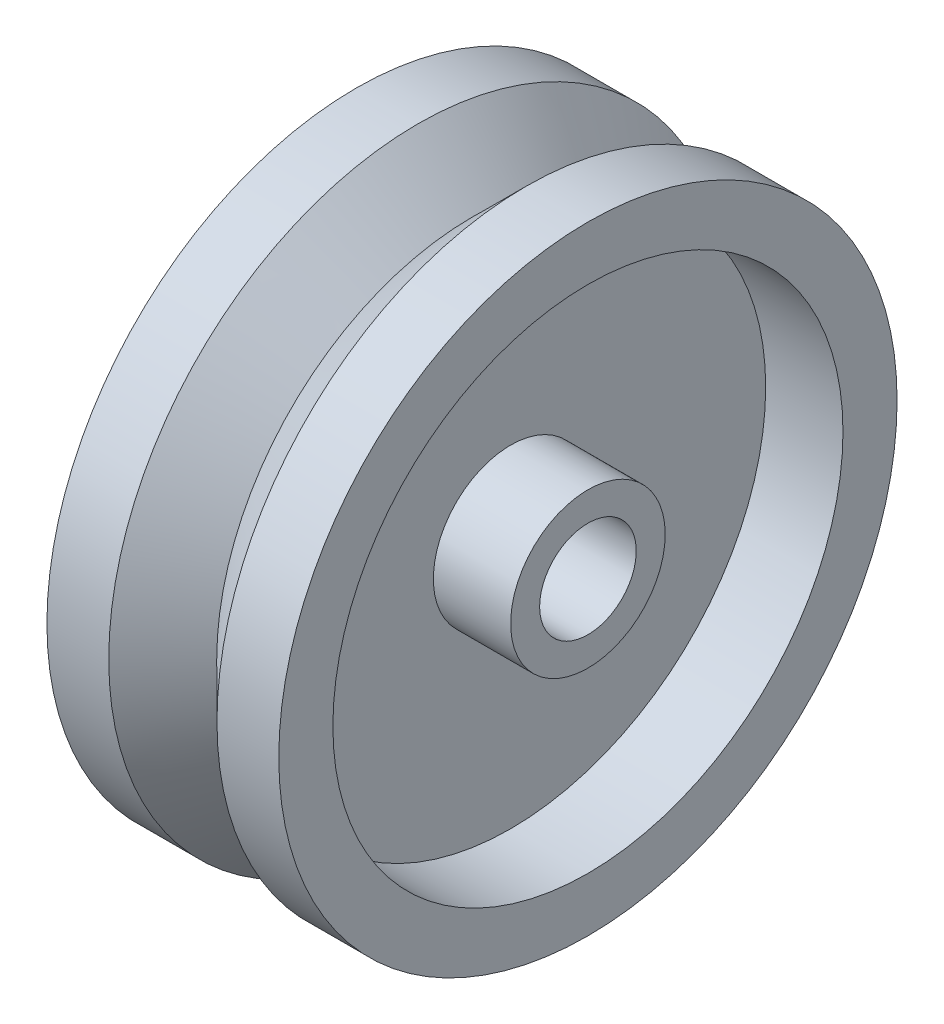
ISO-10303-21;
HEADER;
FILE_DESCRIPTION(('STEP AP214'),'2;1');
FILE_NAME('part.step','',(''),(''),'','','');
FILE_SCHEMA(('AUTOMOTIVE_DESIGN { 1 0 10303 214 1 1 1 1 }'));
ENDSEC;
DATA;
#1=APPLICATION_CONTEXT('core data for automotive mechanical design processes');
#2=APPLICATION_PROTOCOL_DEFINITION('international standard','automotive_design',2000,#1);
#3=PRODUCT_CONTEXT('',#1,'mechanical');
#4=PRODUCT('Part','Part','',(#3));
#5=PRODUCT_RELATED_PRODUCT_CATEGORY('part','',(#4));
#6=PRODUCT_DEFINITION_FORMATION('','',#4);
#7=PRODUCT_DEFINITION_CONTEXT('part definition',#1,'design');
#8=PRODUCT_DEFINITION('design','',#6,#7);
#9=PRODUCT_DEFINITION_SHAPE('','',#8);
#10=(LENGTH_UNIT() NAMED_UNIT(*) SI_UNIT(.MILLI.,.METRE.));
#11=(NAMED_UNIT(*) PLANE_ANGLE_UNIT() SI_UNIT($,.RADIAN.));
#12=(NAMED_UNIT(*) SI_UNIT($,.STERADIAN.) SOLID_ANGLE_UNIT());
#13=UNCERTAINTY_MEASURE_WITH_UNIT(LENGTH_MEASURE(1.E-05),#10,'distance_accuracy_value','');
#14=(GEOMETRIC_REPRESENTATION_CONTEXT(3) GLOBAL_UNCERTAINTY_ASSIGNED_CONTEXT((#13)) GLOBAL_UNIT_ASSIGNED_CONTEXT((#10,
#11,#12)) REPRESENTATION_CONTEXT('',''));
#15=CARTESIAN_POINT('',(0.,0.,0.));
#16=DIRECTION('',(0.,0.,1.));
#17=DIRECTION('',(1.,0.,0.));
#18=AXIS2_PLACEMENT_3D('',#15,#16,#17);
#19=CARTESIAN_POINT('',(-7.5,-3.125,0.));
#20=DIRECTION('',(-1.,0.,0.));
#21=DIRECTION('',(0.,0.,1.));
#22=AXIS2_PLACEMENT_3D('',#19,#20,#21);
#23=PLANE('',#22);
#24=CARTESIAN_POINT('',(-7.5,0.,0.));
#25=DIRECTION('',(-1.,0.,0.));
#26=DIRECTION('',(0.,0.,1.));
#27=AXIS2_PLACEMENT_3D('',#24,#25,#26);
#28=CIRCLE('',#27,3.125);
#29=CARTESIAN_POINT('',(-7.5,0.,3.125));
#30=VERTEX_POINT('',#29);
#31=EDGE_CURVE('E61',#30,#30,#28,.T.);
#32=ORIENTED_EDGE('',*,*,#31,.F.);
#33=EDGE_LOOP('',(#32));
#34=FACE_BOUND('',#33,.T.);
#35=CARTESIAN_POINT('',(-7.5,0.,0.));
#36=DIRECTION('',(1.,0.,0.));
#37=DIRECTION('',(0.,0.,-1.));
#38=AXIS2_PLACEMENT_3D('',#35,#36,#37);
#39=CIRCLE('',#38,5.);
#40=CARTESIAN_POINT('',(-7.5,0.,-5.));
#41=VERTEX_POINT('',#40);
#42=EDGE_CURVE('E84',#41,#41,#39,.T.);
#43=ORIENTED_EDGE('',*,*,#42,.F.);
#44=EDGE_LOOP('',(#43));
#45=FACE_BOUND('',#44,.T.);
#46=ADVANCED_FACE('F40',(#34,#45),#23,.T.);
#47=CARTESIAN_POINT('',(7.5,-3.125,0.));
#48=DIRECTION('',(1.,0.,0.));
#49=DIRECTION('',(0.,0.,-1.));
#50=AXIS2_PLACEMENT_3D('',#47,#48,#49);
#51=PLANE('',#50);
#52=CARTESIAN_POINT('',(7.5,0.,0.));
#53=DIRECTION('',(-1.,0.,0.));
#54=DIRECTION('',(0.,0.,1.));
#55=AXIS2_PLACEMENT_3D('',#52,#53,#54);
#56=CIRCLE('',#55,3.125);
#57=CARTESIAN_POINT('',(7.5,0.,3.125));
#58=VERTEX_POINT('',#57);
#59=EDGE_CURVE('E58',#58,#58,#56,.T.);
#60=ORIENTED_EDGE('',*,*,#59,.T.);
#61=EDGE_LOOP('',(#60));
#62=FACE_BOUND('',#61,.T.);
#63=CARTESIAN_POINT('',(7.5,0.,0.));
#64=DIRECTION('',(1.,0.,0.));
#65=DIRECTION('',(0.,0.,-1.));
#66=AXIS2_PLACEMENT_3D('',#63,#64,#65);
#67=CIRCLE('',#66,5.);
#68=CARTESIAN_POINT('',(7.5,0.,-5.));
#69=VERTEX_POINT('',#68);
#70=EDGE_CURVE('E71',#69,#69,#67,.T.);
#71=ORIENTED_EDGE('',*,*,#70,.T.);
#72=EDGE_LOOP('',(#71));
#73=FACE_BOUND('',#72,.T.);
#74=ADVANCED_FACE('F101',(#62,#73),#51,.T.);
#75=CARTESIAN_POINT('',(-7.5,0.,0.));
#76=DIRECTION('',(1.,0.,0.));
#77=DIRECTION('',(0.,0.,-1.));
#78=AXIS2_PLACEMENT_3D('',#75,#76,#77);
#79=CIRCLE('',#78,16.5);
#80=CARTESIAN_POINT('',(-7.5,0.,-16.5));
#81=VERTEX_POINT('',#80);
#82=EDGE_CURVE('E79',#81,#81,#79,.T.);
#83=ORIENTED_EDGE('',*,*,#82,.T.);
#84=EDGE_LOOP('',(#83));
#85=FACE_BOUND('',#84,.T.);
#86=CARTESIAN_POINT('',(-7.5,0.,0.));
#87=DIRECTION('',(-1.,0.,0.));
#88=DIRECTION('',(0.,0.,1.));
#89=AXIS2_PLACEMENT_3D('',#86,#87,#88);
#90=CIRCLE('',#89,20.);
#91=CARTESIAN_POINT('',(-7.5,0.,20.));
#92=VERTEX_POINT('',#91);
#93=EDGE_CURVE('E10',#92,#92,#90,.T.);
#94=ORIENTED_EDGE('',*,*,#93,.T.);
#95=EDGE_LOOP('',(#94));
#96=FACE_BOUND('',#95,.T.);
#97=ADVANCED_FACE('F39',(#85,#96),#23,.T.);
#98=CARTESIAN_POINT('',(0.,0.,0.));
#99=DIRECTION('',(-1.,0.,0.));
#100=DIRECTION('',(0.,0.,1.));
#101=AXIS2_PLACEMENT_3D('',#98,#99,#100);
#102=CYLINDRICAL_SURFACE('',#101,20.);
#103=CARTESIAN_POINT('',(-3.5,0.,0.));
#104=DIRECTION('',(-1.,0.,0.));
#105=DIRECTION('',(0.,0.,1.));
#106=AXIS2_PLACEMENT_3D('',#103,#104,#105);
#107=CIRCLE('',#106,20.);
#108=CARTESIAN_POINT('',(-3.5,0.,20.));
#109=VERTEX_POINT('',#108);
#110=EDGE_CURVE('E42',#109,#109,#107,.T.);
#111=ORIENTED_EDGE('',*,*,#110,.T.);
#112=EDGE_LOOP('',(#111));
#113=FACE_BOUND('',#112,.T.);
#114=ORIENTED_EDGE('',*,*,#93,.F.);
#115=EDGE_LOOP('',(#114));
#116=FACE_BOUND('',#115,.T.);
#117=ADVANCED_FACE('F115',(#113,#116),#102,.T.);
#118=CARTESIAN_POINT('',(-3.5,0.,0.));
#119=DIRECTION('',(-1.,0.,0.));
#120=DIRECTION('',(0.,0.,1.));
#121=AXIS2_PLACEMENT_3D('',#118,#119,#120);
#122=CONICAL_SURFACE('',#121,20.,0.783281559458102);
#123=CARTESIAN_POINT('',(0.,0.,0.));
#124=DIRECTION('',(-1.,0.,0.));
#125=DIRECTION('',(0.,0.,1.));
#126=AXIS2_PLACEMENT_3D('',#123,#124,#125);
#127=CIRCLE('',#126,16.5147849557588);
#128=CARTESIAN_POINT('',(0.,0.,16.5147849557588));
#129=VERTEX_POINT('',#128);
#130=EDGE_CURVE('E48',#129,#129,#127,.T.);
#131=ORIENTED_EDGE('',*,*,#130,.T.);
#132=EDGE_LOOP('',(#131));
#133=FACE_BOUND('',#132,.T.);
#134=ORIENTED_EDGE('',*,*,#110,.F.);
#135=EDGE_LOOP('',(#134));
#136=FACE_BOUND('',#135,.T.);
#137=ADVANCED_FACE('F116',(#133,#136),#122,.T.);
#138=CARTESIAN_POINT('',(0.,0.,0.));
#139=DIRECTION('',(1.,0.,0.));
#140=DIRECTION('',(0.,0.,-1.));
#141=AXIS2_PLACEMENT_3D('',#138,#139,#140);
#142=CONICAL_SURFACE('',#141,16.5147849557588,0.783281559458103);
#143=CARTESIAN_POINT('',(3.5,0.,0.));
#144=DIRECTION('',(-1.,0.,0.));
#145=DIRECTION('',(0.,0.,1.));
#146=AXIS2_PLACEMENT_3D('',#143,#144,#145);
#147=CIRCLE('',#146,20.);
#148=CARTESIAN_POINT('',(3.5,0.,20.));
#149=VERTEX_POINT('',#148);
#150=EDGE_CURVE('E55',#149,#149,#147,.T.);
#151=ORIENTED_EDGE('',*,*,#150,.T.);
#152=EDGE_LOOP('',(#151));
#153=FACE_BOUND('',#152,.T.);
#154=ORIENTED_EDGE('',*,*,#130,.F.);
#155=EDGE_LOOP('',(#154));
#156=FACE_BOUND('',#155,.T.);
#157=ADVANCED_FACE('F149',(#153,#156),#142,.T.);
#158=CARTESIAN_POINT('',(0.,0.,0.));
#159=DIRECTION('',(-1.,0.,0.));
#160=DIRECTION('',(0.,0.,1.));
#161=AXIS2_PLACEMENT_3D('',#158,#159,#160);
#162=CYLINDRICAL_SURFACE('',#161,20.);
#163=CARTESIAN_POINT('',(7.5,0.,0.));
#164=DIRECTION('',(-1.,0.,0.));
#165=DIRECTION('',(0.,0.,1.));
#166=AXIS2_PLACEMENT_3D('',#163,#164,#165);
#167=CIRCLE('',#166,20.);
#168=CARTESIAN_POINT('',(7.5,0.,20.));
#169=VERTEX_POINT('',#168);
#170=EDGE_CURVE('E60',#169,#169,#167,.T.);
#171=ORIENTED_EDGE('',*,*,#170,.T.);
#172=EDGE_LOOP('',(#171));
#173=FACE_BOUND('',#172,.T.);
#174=ORIENTED_EDGE('',*,*,#150,.F.);
#175=EDGE_LOOP('',(#174));
#176=FACE_BOUND('',#175,.T.);
#177=ADVANCED_FACE('F144',(#173,#176),#162,.T.);
#178=CARTESIAN_POINT('',(7.5,0.,0.));
#179=DIRECTION('',(1.,0.,0.));
#180=DIRECTION('',(0.,0.,-1.));
#181=AXIS2_PLACEMENT_3D('',#178,#179,#180);
#182=CIRCLE('',#181,16.5);
#183=CARTESIAN_POINT('',(7.5,0.,-16.5));
#184=VERTEX_POINT('',#183);
#185=EDGE_CURVE('E70',#184,#184,#182,.T.);
#186=ORIENTED_EDGE('',*,*,#185,.F.);
#187=EDGE_LOOP('',(#186));
#188=FACE_BOUND('',#187,.T.);
#189=ORIENTED_EDGE('',*,*,#170,.F.);
#190=EDGE_LOOP('',(#189));
#191=FACE_BOUND('',#190,.T.);
#192=ADVANCED_FACE('F109',(#188,#191),#51,.T.);
#193=CARTESIAN_POINT('',(0.,0.,0.));
#194=DIRECTION('',(-1.,0.,0.));
#195=DIRECTION('',(0.,0.,1.));
#196=AXIS2_PLACEMENT_3D('',#193,#194,#195);
#197=CYLINDRICAL_SURFACE('',#196,3.125);
#198=ORIENTED_EDGE('',*,*,#31,.T.);
#199=EDGE_LOOP('',(#198));
#200=FACE_BOUND('',#199,.T.);
#201=ORIENTED_EDGE('',*,*,#59,.F.);
#202=EDGE_LOOP('',(#201));
#203=FACE_BOUND('',#202,.T.);
#204=ADVANCED_FACE('F138',(#200,#203),#197,.F.);
#205=CARTESIAN_POINT('',(2.5,0.,0.));
#206=DIRECTION('',(1.,0.,0.));
#207=DIRECTION('',(0.,0.,-1.));
#208=AXIS2_PLACEMENT_3D('',#205,#206,#207);
#209=CYLINDRICAL_SURFACE('',#208,16.5);
#210=CARTESIAN_POINT('',(2.5,0.,0.));
#211=DIRECTION('',(1.,0.,0.));
#212=DIRECTION('',(0.,0.,-1.));
#213=AXIS2_PLACEMENT_3D('',#210,#211,#212);
#214=CIRCLE('',#213,16.5);
#215=CARTESIAN_POINT('',(2.5,0.,-16.5));
#216=VERTEX_POINT('',#215);
#217=EDGE_CURVE('E66',#216,#216,#214,.T.);
#218=ORIENTED_EDGE('',*,*,#217,.F.);
#219=EDGE_LOOP('',(#218));
#220=FACE_BOUND('',#219,.T.);
#221=ORIENTED_EDGE('',*,*,#185,.T.);
#222=EDGE_LOOP('',(#221));
#223=FACE_BOUND('',#222,.T.);
#224=ADVANCED_FACE('F132',(#220,#223),#209,.F.);
#225=CARTESIAN_POINT('',(2.5,0.,0.));
#226=DIRECTION('',(1.,0.,0.));
#227=DIRECTION('',(0.,0.,-1.));
#228=AXIS2_PLACEMENT_3D('',#225,#226,#227);
#229=PLANE('',#228);
#230=CARTESIAN_POINT('',(2.5,0.,0.));
#231=DIRECTION('',(1.,0.,0.));
#232=DIRECTION('',(0.,0.,-1.));
#233=AXIS2_PLACEMENT_3D('',#230,#231,#232);
#234=CIRCLE('',#233,5.);
#235=CARTESIAN_POINT('',(2.5,0.,-5.));
#236=VERTEX_POINT('',#235);
#237=EDGE_CURVE('E69',#236,#236,#234,.T.);
#238=ORIENTED_EDGE('',*,*,#237,.F.);
#239=EDGE_LOOP('',(#238));
#240=FACE_BOUND('',#239,.T.);
#241=ORIENTED_EDGE('',*,*,#217,.T.);
#242=EDGE_LOOP('',(#241));
#243=FACE_BOUND('',#242,.T.);
#244=ADVANCED_FACE('F133',(#240,#243),#229,.T.);
#245=CARTESIAN_POINT('',(2.5,0.,0.));
#246=DIRECTION('',(1.,0.,0.));
#247=DIRECTION('',(0.,0.,-1.));
#248=AXIS2_PLACEMENT_3D('',#245,#246,#247);
#249=CYLINDRICAL_SURFACE('',#248,5.);
#250=ORIENTED_EDGE('',*,*,#237,.T.);
#251=EDGE_LOOP('',(#250));
#252=FACE_BOUND('',#251,.T.);
#253=ORIENTED_EDGE('',*,*,#70,.F.);
#254=EDGE_LOOP('',(#253));
#255=FACE_BOUND('',#254,.T.);
#256=ADVANCED_FACE('F127',(#252,#255),#249,.T.);
#257=CARTESIAN_POINT('',(-2.5,0.,0.));
#258=DIRECTION('',(-1.,0.,0.));
#259=DIRECTION('',(0.,0.,-1.));
#260=AXIS2_PLACEMENT_3D('',#257,#258,#259);
#261=PLANE('',#260);
#262=CARTESIAN_POINT('',(-2.5,0.,0.));
#263=DIRECTION('',(1.,0.,0.));
#264=DIRECTION('',(0.,0.,-1.));
#265=AXIS2_PLACEMENT_3D('',#262,#263,#264);
#266=CIRCLE('',#265,16.5);
#267=CARTESIAN_POINT('',(-2.5,0.,-16.5));
#268=VERTEX_POINT('',#267);
#269=EDGE_CURVE('E78',#268,#268,#266,.T.);
#270=ORIENTED_EDGE('',*,*,#269,.F.);
#271=EDGE_LOOP('',(#270));
#272=FACE_BOUND('',#271,.T.);
#273=CARTESIAN_POINT('',(-2.5,0.,0.));
#274=DIRECTION('',(1.,0.,0.));
#275=DIRECTION('',(0.,0.,-1.));
#276=AXIS2_PLACEMENT_3D('',#273,#274,#275);
#277=CIRCLE('',#276,5.);
#278=CARTESIAN_POINT('',(-2.5,0.,-5.));
#279=VERTEX_POINT('',#278);
#280=EDGE_CURVE('E85',#279,#279,#277,.T.);
#281=ORIENTED_EDGE('',*,*,#280,.T.);
#282=EDGE_LOOP('',(#281));
#283=FACE_BOUND('',#282,.T.);
#284=ADVANCED_FACE('F93',(#272,#283),#261,.T.);
#285=CARTESIAN_POINT('',(-2.5,0.,0.));
#286=DIRECTION('',(-1.,0.,0.));
#287=DIRECTION('',(0.,0.,1.));
#288=AXIS2_PLACEMENT_3D('',#285,#286,#287);
#289=CYLINDRICAL_SURFACE('',#288,16.5);
#290=ORIENTED_EDGE('',*,*,#269,.T.);
#291=EDGE_LOOP('',(#290));
#292=FACE_BOUND('',#291,.T.);
#293=ORIENTED_EDGE('',*,*,#82,.F.);
#294=EDGE_LOOP('',(#293));
#295=FACE_BOUND('',#294,.T.);
#296=ADVANCED_FACE('F96',(#292,#295),#289,.F.);
#297=CARTESIAN_POINT('',(-2.5,0.,0.));
#298=DIRECTION('',(-1.,0.,0.));
#299=DIRECTION('',(0.,0.,1.));
#300=AXIS2_PLACEMENT_3D('',#297,#298,#299);
#301=CYLINDRICAL_SURFACE('',#300,5.);
#302=ORIENTED_EDGE('',*,*,#280,.F.);
#303=EDGE_LOOP('',(#302));
#304=FACE_BOUND('',#303,.T.);
#305=ORIENTED_EDGE('',*,*,#42,.T.);
#306=EDGE_LOOP('',(#305));
#307=FACE_BOUND('',#306,.T.);
#308=ADVANCED_FACE('F91',(#304,#307),#301,.T.);
#309=CLOSED_SHELL('',(#46,#74,#97,#117,#137,#157,#177,#192,#204,#224,#244,#256,#284,#296,#308));
#310=MANIFOLD_SOLID_BREP('B2',#309);
#311=ADVANCED_BREP_SHAPE_REPRESENTATION('',(#18,#310),#14);
#312=SHAPE_DEFINITION_REPRESENTATION(#9,#311);
ENDSEC;
END-ISO-10303-21;
